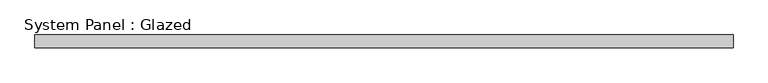
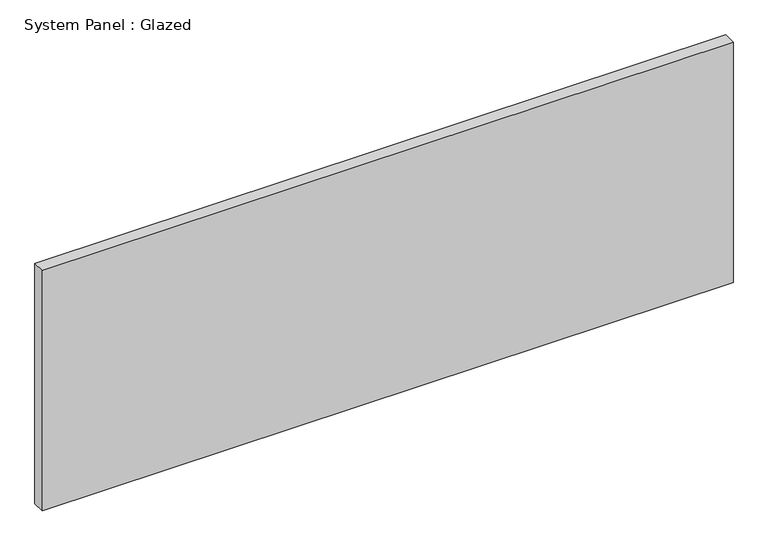
"""IFC4 building model written with IfcOpenShell, lengths in millimetres: plate geometry, System Panel : Glazed."""

from ifc_helpers import new_model, si_unit, origin, origin_with_axes, place, context, project, spatial, polyline, outline, extrude, source, transform, mapped, element, save


def system_panel_glazed_9470322e(model_context):
    return source(origin(), model_context, "Body", "SweptSolid", [
        extrude(outline(polyline([(698.6142406, -44.45), (-698.6142406, -44.45), (-698.6142406, -19.05), (698.6142406, -19.05), (698.6142406, -44.45)])), origin_with_axes(), (0.0, 0.0, 1.0), 514.35),
    ])


if __name__ == "__main__":
    model = new_model("IFC4")
    model_context = context("Model", 3, world=origin())
    ifc_project = project(units=[si_unit("LENGTHUNIT", "METRE", prefix="MILLI")], contexts=[model_context])
    site = spatial("IfcSite", under=ifc_project)
    building = spatial("IfcBuilding", under=site)
    placement = place(None, origin())
    system_panel_glazed_shape = system_panel_glazed_9470322e(model_context)
    element("IfcPlate", 1, ObjectType="System Panel : Glazed", at=placement, inside=building, context=model_context, shape_type="MappedRepresentation", body=[
        mapped(system_panel_glazed_shape, transform((0.0, 0.0, 0.0), x_axis=(1.0, 0.0, 0.0), y_axis=(0.0, 1.0, 0.0), z_axis=(0.0, 0.0, 1.0))),
    ])
    save(model, "model.ifc")

# Revit data of these elements
# Type "System Panel : Glazed"
#   Construction Type Id = "GSP4R"
#   Analytic Construction = "1/8 in Pilkington single glazing"
#   Visual Light Transmittance = 0.9
#   Solar Heat Gain Coefficient = 0.86
#   Heat Transfer Coefficient (U) = 1.18115 BTU/(h·ft²·°F)
#   Define Thermal Properties by = 1
# Element 1 (IfcPlate, "System Panel : Glazed")
#   Materials on its faces: "glass panel 223"
# Materials
#   "glass panel 223": class "Generic", colour RGB 120 120 120, transparency 0, Cost = 0
